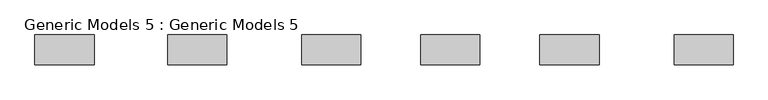
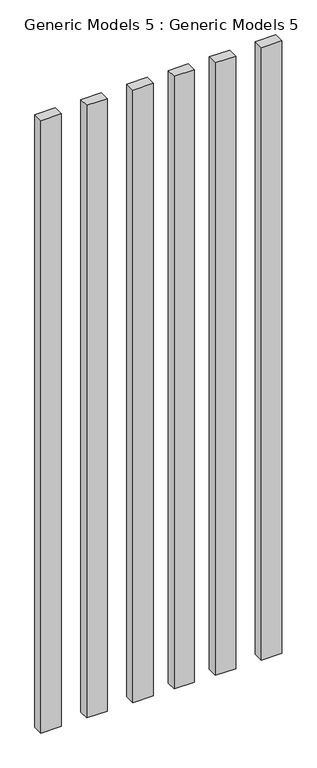
"""IFC4 building model written with IfcOpenShell, lengths in millimetres: proxy geometry, Generic Models 5 : Generic Models 5."""

from ifc_helpers import new_model, si_unit, frame, origin, place, context, project, spatial, polyline, outline, extrude, source, transform, mapped, element, save


def generic_models_5_generic_models_5_60d6e435(model_context):
    return source(origin(), model_context, "Body", "SweptSolid", [
        extrude(outline(polyline([(-19013.3920853, -4379.8846041), (-19013.3920853, -4430.6846041), (-19114.9920853, -4430.6846041), (-19114.9920853, -4379.8846041), (-19013.3920853, -4379.8846041)])), frame((0.0, 0.0, 3505.2), z_axis=(0.0, 0.0, 1.0), x_axis=(1.0, 0.0, 0.0)), (0.0, 0.0, 1.0), 3200.4),
        extrude(outline(polyline([(-18787.7570066, -4379.8846041), (-18787.7570066, -4430.6846041), (-18888.5393817, -4430.6846041), (-18888.5393817, -4379.8846041), (-18787.7570066, -4379.8846041)])), frame((0.0, 0.0, 3505.2), z_axis=(0.0, 0.0, 1.0), x_axis=(1.0, 0.0, 0.0)), (0.0, 0.0, 1.0), 3200.4),
        extrude(outline(polyline([(-18559.1570066, -4379.8846041), (-18559.1570066, -4430.6846041), (-18659.9393817, -4430.6846041), (-18659.9393817, -4379.8846041), (-18559.1570066, -4379.8846041)])), frame((0.0, 0.0, 3505.2), z_axis=(0.0, 0.0, 1.0), x_axis=(1.0, 0.0, 0.0)), (0.0, 0.0, 1.0), 3200.4),
        extrude(outline(polyline([(-18355.9570066, -4379.8846041), (-18355.9570066, -4430.6846041), (-18456.7393817, -4430.6846041), (-18456.7393817, -4379.8846041), (-18355.9570066, -4379.8846041)])), frame((0.0, 0.0, 3505.2), z_axis=(0.0, 0.0, 1.0), x_axis=(1.0, 0.0, 0.0)), (0.0, 0.0, 1.0), 3200.4),
        extrude(outline(polyline([(-18152.7570066, -4379.8846041), (-18152.7570066, -4430.6846041), (-18253.5393817, -4430.6846041), (-18253.5393817, -4379.8846041), (-18152.7570066, -4379.8846041)])), frame((0.0, 0.0, 3505.2), z_axis=(0.0, 0.0, 1.0), x_axis=(1.0, 0.0, 0.0)), (0.0, 0.0, 1.0), 3200.4),
        extrude(outline(polyline([(-17924.1570066, -4379.8846041), (-17924.1570066, -4430.6846041), (-18024.9393817, -4430.6846041), (-18024.9393817, -4379.8846041), (-17924.1570066, -4379.8846041)])), frame((0.0, 0.0, 3505.2), z_axis=(0.0, 0.0, 1.0), x_axis=(1.0, 0.0, 0.0)), (0.0, 0.0, 1.0), 3200.4),
    ])


if __name__ == "__main__":
    model = new_model("IFC4")
    model_context = context("Model", 3, world=origin())
    ifc_project = project(units=[si_unit("LENGTHUNIT", "METRE", prefix="MILLI")], contexts=[model_context])
    site = spatial("IfcSite", under=ifc_project)
    building = spatial("IfcBuilding", under=site)
    placement = place(None, origin())
    generic_models_5_generic_models_5_shape = generic_models_5_generic_models_5_60d6e435(model_context)
    element("IfcBuildingElementProxy", 1, Name="Generic Models 5 : Generic Models 5", ObjectType="Generic Models 5 : Generic Models 5", at=placement, inside=building, context=model_context, shape_type="MappedRepresentation", body=[
        mapped(generic_models_5_generic_models_5_shape, transform((0.0, 0.0, 0.0), x_axis=(1.0, 0.0, 0.0), y_axis=(0.0, 1.0, 0.0), z_axis=(0.0, 0.0, 1.0))),
    ])
    save(model, "model.ifc")
